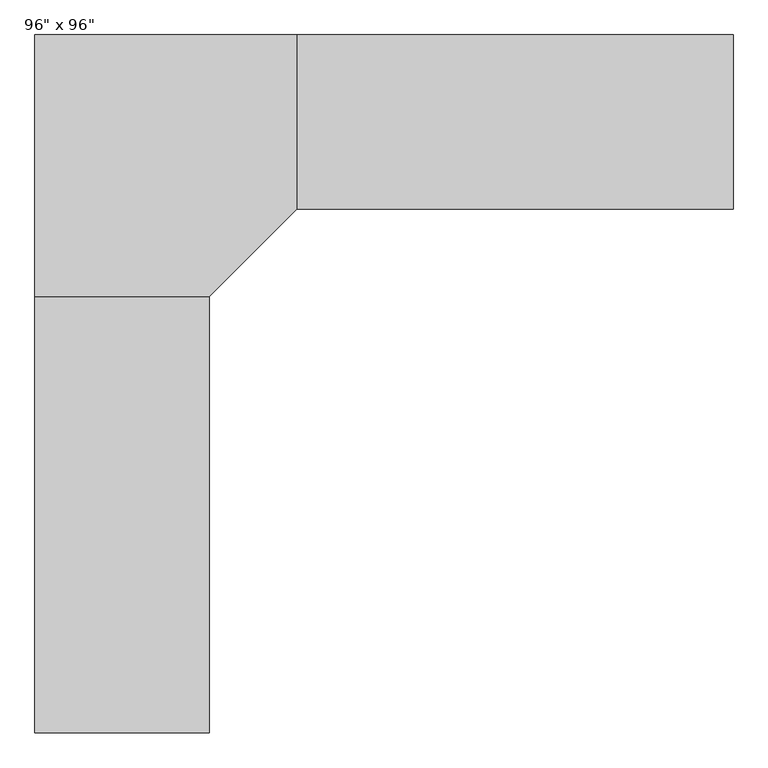
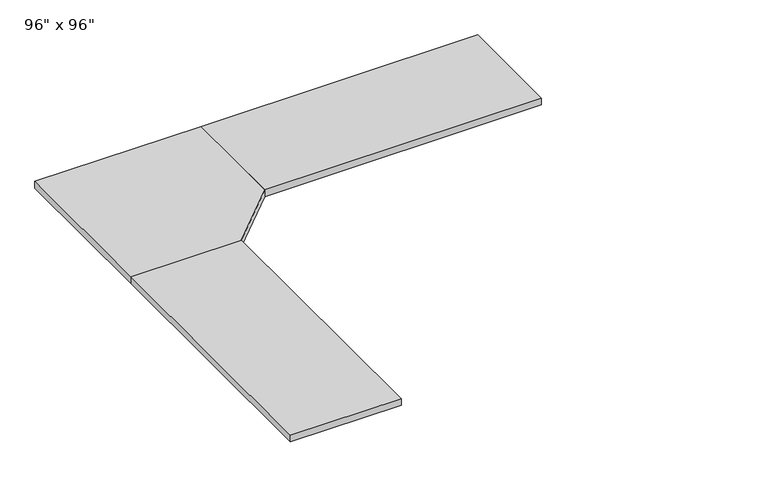
"""IFC4 building model written with IfcOpenShell, lengths in millimetres: furniture geometry."""

from ifc_helpers import new_model, si_unit, frame, origin, place, context, project, spatial, polyline, outline, extrude, source, transform, mapped, element, save


def furniture_07436f11(model_context):
    return source(origin(), model_context, "Body", "SweptSolid", [
        extrude(outline(polyline([(-80.9317522, -545.8230076), (833.4682478, -545.8230076), (833.4682478, -1155.4230076), (528.6682478, -1460.2230076), (-80.9317522, -1460.2230076), (-80.9317522, -545.8230076)])), frame((0.0, 0.0, 723.9), z_axis=(0.0, 0.0, 1.0), x_axis=(1.0, 0.0, 0.0)), (0.0, 0.0, 1.0), 38.1),
        extrude(outline(polyline([(528.6682478, -2984.2230076), (-80.9317522, -2984.2230076), (-80.9317522, -1460.2230076), (528.6682478, -1460.2230076), (528.6682478, -2984.2230076)])), frame((0.0, 0.0, 723.9), z_axis=(0.0, 0.0, 1.0), x_axis=(1.0, 0.0, 0.0)), (0.0, 0.0, 1.0), 38.1),
        extrude(outline(polyline([(2357.4682478, -1155.4230076), (833.4682478, -1155.4230076), (833.4682478, -545.8230076), (2357.4682478, -545.8230076), (2357.4682478, -1155.4230076)])), frame((0.0, 0.0, 723.9), z_axis=(0.0, 0.0, 1.0), x_axis=(1.0, 0.0, 0.0)), (0.0, 0.0, 1.0), 38.1),
    ])


if __name__ == "__main__":
    model = new_model("IFC4")
    model_context = context("Model", 3, world=origin())
    ifc_project = project(units=[si_unit("LENGTHUNIT", "METRE", prefix="MILLI")], contexts=[model_context])
    site = spatial("IfcSite", under=ifc_project)
    building = spatial("IfcBuilding", under=site)
    placement = place(None, origin())
    furniture_shape = furniture_07436f11(model_context)
    element("IfcFurniture", 1, ObjectType="96\" x 96\"", at=placement, inside=building, context=model_context, shape_type="MappedRepresentation", body=[
        mapped(furniture_shape, transform((0.0, 0.0, 0.0), x_axis=(1.0, 0.0, 0.0), y_axis=(0.0, 1.0, 0.0), z_axis=(0.0, 0.0, 1.0))),
    ])
    save(model, "model.ifc")

# Revit data of these elements
# Type "96\" x 96\""
#   Assembly Code = "E2020"
#   Desktop Height = 2' - 6"
#   Desktop1 Width = 2' - 0"
#   Desktop2 Width = 2' - 0"
#   Panel1 Length = 5' - 0"
#   Panel2 Length = 5' - 0"
#   Work Top Material = Laminate, Ivory, Matte
#   Default Elevation = 0
# Element 1 (IfcFurniture, "96\" x 96\"")
#   Materials on its faces: "Laminate, Ivory, Matte"
# Materials
#   "Laminate, Ivory, Matte": class "Plastic", colour RGB 247 247 239, transparency 0, Description = "Plastic Laminate - Ivory, Matte", Cost = 0
